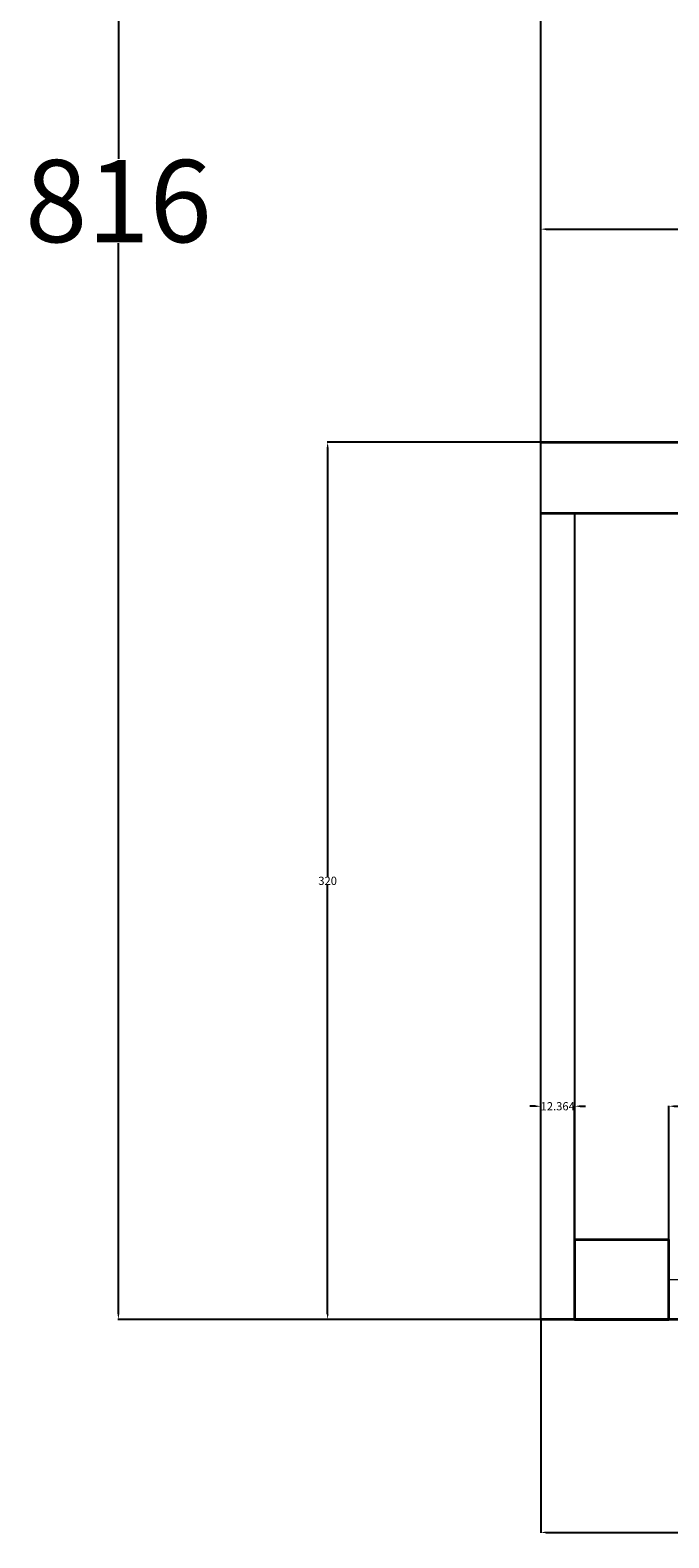
# Model space of a CAD drawing. Units: centimetres. Extents: x -121 to 3851, y -16 to 1180.
# Tile 10 of 16: x 2225 to 2458, y 16 to 566. Entities that reach past the tile are written whole.
import ezdxf

# ---------------------------------------------------------------- set-up
doc = ezdxf.new("R2010")
doc.units = ezdxf.units.CM
doc.header["$MEASUREMENT"] = 0
for name, color, linetype, lineweight in [('A-ANNO-DIMS', 2, 'Continuous', 18), ('A-COLS', 7, 'Continuous', 35), ('A-FLOR', 8, 'Continuous', 25), ('A-FLOR-HRAL', 4, 'Continuous', 18), ('A-WALL', 7, 'Continuous', 35)]:
    doc.layers.add(name, color=color, linetype=linetype, lineweight=lineweight)
doc.styles.get("Standard").update_dxf_attribs({"font": 'arial.ttf'})
doc.dimstyles.get("Standard").update_dxf_attribs({"dimtxt": 3, "dimasz": 2, "dimexe": 0.18, "dimexo": 0.0625, "dimgap": 0.09, "dimtad": 0, "dimtih": 1, "dimtoh": 1, "dimdec": 0, "dimzin": 0, "dimdsep": 46, "dimtxsty": 'Standard', "dimcen": 0.09, "dimadec": 0, "dimazin": 0, "dimtfac": 1, "dimtdec": 0, "dimtofl": 0, "dimtmove": 0, "dimatfit": 3, "dimfxl": 1, "dimtolj": 1, "dimtzin": 0, "dimarcsym": 0})

# ---------------------------------------------------------------- blocks, each defined once
blk = doc.blocks.new('*D13')
at = {"layer": 'A-ANNO-DIMS', "color": 0, "lineweight": -2, "transparency": 16777216}
for p, q in [((2411.2, 911.72), (2257.01, 911.72)), ((2257.19, 909.72), (2257.19, 519.13)), ((2257.19, 97.72), (2257.19, 488.32)), ((2411.2, 95.72), (2257.01, 95.72))]:
    blk.add_line(p, q, dxfattribs=at)
at = {"layer": 'A-ANNO-DIMS', "color": 0, "transparency": 16777216}
for points in [[(2256.85, 909.72), (2257.52, 909.72), (2257.19, 911.72)], [(2256.85, 97.72), (2257.52, 97.72), (2257.19, 95.72)]]:
    blk.add_solid(points, dxfattribs=at)
at = {"layer": 'Defpoints', "color": 0, "transparency": 16777216}
for p in [(2411.26, 911.72), (2257.19, 95.72), (2411.26, 95.72)]:
    blk.add_point(p, dxfattribs=at)
at = {"layer": 'A-ANNO-DIMS', "color": 0, "transparency": 16777216, "insert": (2257.19, 503.72), "char_height": 3, "attachment_point": 5}
blk.add_mtext('\\A1;{\\H10x;816}', dxfattribs=at)
blk = doc.blocks.new('POST-34X29CM')
blk.add_lwpolyline([(0, 0), (34.36, 0), (34.36, 28.96), (0, 28.96)], close=True)
blk = doc.blocks.new('*D66')
at = {"layer": 'A-ANNO-DIMS', "color": 0, "lineweight": -2, "transparency": 16777216}
for p, q in [((2411.2, 415.72), (2333.33, 415.72)), ((2333.51, 413.72), (2333.51, 257.35)), ((2333.51, 97.72), (2333.51, 254.1)), ((2411.2, 95.72), (2333.33, 95.72))]:
    blk.add_line(p, q, dxfattribs=at)
at = {"layer": 'A-ANNO-DIMS', "color": 0, "transparency": 16777216}
for points in [[(2333.18, 413.72), (2333.85, 413.72), (2333.51, 415.72)], [(2333.18, 97.72), (2333.85, 97.72), (2333.51, 95.72)]]:
    blk.add_solid(points, dxfattribs=at)
at = {"layer": 'Defpoints', "color": 0, "transparency": 16777216}
for p in [(2411.26, 415.72), (2333.51, 95.72), (2411.26, 95.72)]:
    blk.add_point(p, dxfattribs=at)
at = {"layer": 'A-ANNO-DIMS', "color": 0, "transparency": 16777216, "insert": (2333.51, 255.72), "char_height": 3, "attachment_point": 5}
blk.add_mtext('\\A1;320', dxfattribs=at)
blk = doc.blocks.new('*D67')
at = {"layer": 'A-ANNO-DIMS', "color": 0, "lineweight": -2, "transparency": 16777216}
for p, q in [((2411.26, 95.66), (2411.26, 17.79)), ((2821.26, 95.66), (2821.26, 17.79)), ((2413.26, 17.97), (2612.8, 17.97)), ((2819.26, 17.97), (2619.72, 17.97))]:
    blk.add_line(p, q, dxfattribs=at)
at = {"layer": 'A-ANNO-DIMS', "color": 0, "transparency": 16777216}
for points in [[(2413.26, 18.31), (2413.26, 17.64), (2411.26, 17.97)], [(2819.26, 18.31), (2819.26, 17.64), (2821.26, 17.97)]]:
    blk.add_solid(points, dxfattribs=at)
at = {"layer": 'Defpoints', "color": 0, "transparency": 16777216}
for p in [(2411.26, 95.72), (2821.26, 95.72), (2821.26, 17.97)]:
    blk.add_point(p, dxfattribs=at)
at = {"layer": 'A-ANNO-DIMS', "color": 0, "transparency": 16777216, "insert": (2616.26, 17.97), "char_height": 3, "attachment_point": 5}
blk.add_mtext('\\A1;410', dxfattribs=at)
blk = doc.blocks.new('*D75')
at = {"layer": 'A-ANNO-DIMS', "color": 0, "lineweight": -2, "transparency": 16777216}
for p, q in [((2409.26, 173.47), (2407.26, 173.47)), ((2411.26, 95.79), (2411.26, 173.65)), ((2423.63, 95.79), (2423.63, 173.65)), ((2425.63, 173.47), (2427.63, 173.47))]:
    blk.add_line(p, q, dxfattribs=at)
at = {"layer": 'A-ANNO-DIMS', "color": 0, "transparency": 16777216}
for points in [[(2409.26, 173.81), (2409.26, 173.14), (2411.26, 173.47)], [(2425.63, 173.81), (2425.63, 173.14), (2423.63, 173.47)]]:
    blk.add_solid(points, dxfattribs=at)
at = {"layer": 'Defpoints', "color": 0, "transparency": 16777216}
for p in [(2423.63, 173.47), (2411.26, 95.72), (2423.63, 95.72)]:
    blk.add_point(p, dxfattribs=at)
at = {"layer": 'A-ANNO-DIMS', "color": 0, "transparency": 16777216, "insert": (2417.45, 173.47), "char_height": 3, "attachment_point": 5}
blk.add_mtext('\\A1;12.364', dxfattribs=at)
blk = doc.blocks.new('*D76')
at = {"layer": 'A-ANNO-DIMS', "color": 0, "lineweight": -2, "transparency": 16777216}
for p, q in [((2457.99, 95.79), (2457.99, 173.65)), ((2459.99, 173.47), (2519.59, 173.47)), ((2591.55, 173.47), (2531.94, 173.47)), ((2593.55, 95.79), (2593.55, 173.65))]:
    blk.add_line(p, q, dxfattribs=at)
at = {"layer": 'A-ANNO-DIMS', "color": 0, "transparency": 16777216}
for points in [[(2459.99, 173.81), (2459.99, 173.14), (2457.99, 173.47)], [(2591.55, 173.81), (2591.55, 173.14), (2593.55, 173.47)]]:
    blk.add_solid(points, dxfattribs=at)
at = {"layer": 'Defpoints', "color": 0, "transparency": 16777216}
for p in [(2593.55, 173.47), (2457.99, 95.72), (2593.55, 95.72)]:
    blk.add_point(p, dxfattribs=at)
at = {"layer": 'A-ANNO-DIMS', "color": 0, "transparency": 16777216, "insert": (2525.77, 173.47), "char_height": 3, "attachment_point": 5}
blk.add_mtext('\\A1;135.56', dxfattribs=at)
blk = doc.blocks.new('*D78')
at = {"layer": 'A-ANNO-DIMS', "color": 0, "lineweight": -2, "transparency": 16777216}
for p, q in [((2411.26, 415.79), (2411.26, 493.65)), ((2413.26, 493.47), (2538, 493.47)), ((2675.4, 493.47), (2550.67, 493.47)), ((2677.4, 415.79), (2677.4, 493.65))]:
    blk.add_line(p, q, dxfattribs=at)
at = {"layer": 'A-ANNO-DIMS', "color": 0, "transparency": 16777216}
for points in [[(2413.26, 493.81), (2413.26, 493.14), (2411.26, 493.47)], [(2675.4, 493.81), (2675.4, 493.14), (2677.4, 493.47)]]:
    blk.add_solid(points, dxfattribs=at)
at = {"layer": 'Defpoints', "color": 0, "transparency": 16777216}
for p in [(2677.4, 493.47), (2411.26, 415.72), (2677.4, 415.72)]:
    blk.add_point(p, dxfattribs=at)
at = {"layer": 'A-ANNO-DIMS', "color": 0, "transparency": 16777216, "insert": (2544.33, 493.47), "char_height": 3, "attachment_point": 5}
blk.add_mtext('\\A1;266.14', dxfattribs=at)

msp = doc.modelspace()

# ---------------------------------------------------------------- linework, layer by layer
at = {"layer": 'A-FLOR'}
for p, q in [((2411.2642, 95.7228), (2411.2642, 911.7228)), ((2423.6282, 389.7228), (2423.6282, 95.7228))]:
    msp.add_line(p, q, dxfattribs=at)
at = {"layer": 'A-FLOR-HRAL'}
msp.add_line((2457.9883, 110.2005), (2593.5502, 111.1316), dxfattribs=at)
at = {"layer": 'A-WALL'}
for p, q in [((2411.2642, 415.7228), (2677.3995, 415.7228)), ((2661.5376, 389.7228), (2411.2642, 389.7228)), ((3767.2642, 95.7228), (2411.2642, 95.7228))]:
    msp.add_line(p, q, dxfattribs=at)

# ---------------------------------------------------------------- block references
at = {"layer": 'A-COLS'}
msp.add_blockref('POST-34X29CM', (2423.628, 95.7227), dxfattribs=at)

# ---------------------------------------------------------------- dimensions: what is measured, and where the dimension line sits
at = {"layer": 'A-ANNO-DIMS'}
dim = msp.add_linear_dim(base=(2257.1851, 95.7228), p1=(2411.2642, 911.7228), p2=(2411.2642, 95.7228), angle=90, text='{\\H10x;<>}', dimstyle='Standard', override={"dimclrd": 0, "dimclre": 0, "dimclrt": 0}, dxfattribs=at)
dim.commit()
dim.dimension.update_dxf_attribs({"geometry": '*D13', "text_midpoint": (2257.1851, 503.7228)})
for base, p1, p2, override, picture, middle in [((2677.3995, 493.4728), (2411.2642, 415.7228), (2677.3995, 415.7228), {"dimdec": 2, "dimlfac": 1, "dimrnd": 0, "dimzin": 0, "dimdsep": 46, "dimlunit": 2}, '*D78', (2544.3319, 493.4728)), ((2423.6282, 173.4728), (2411.2642, 95.7228), (2423.6282, 95.7228), {"dimdec": 3, "dimlfac": 1, "dimrnd": 0, "dimzin": 0, "dimdsep": 46, "dimlunit": 2}, '*D75', (2417.4462, 173.4728)), ((2593.5502, 173.4728), (2457.9883, 95.7228), (2593.5502, 95.7228), {"dimdec": 2, "dimlfac": 1, "dimrnd": 0, "dimzin": 0, "dimdsep": 46, "dimlunit": 2}, '*D76', (2525.7693, 173.4728)), ((2821.2642, 17.9728), (2411.2642, 95.7228), (2821.2642, 95.7228), {"dimdec": 0, "dimlfac": 1, "dimrnd": 0, "dimzin": 0, "dimdsep": 46, "dimlunit": 2}, '*D67', (2616.2642, 17.9728))]:
    dim = msp.add_linear_dim(base=base, p1=p1, p2=p2, dimstyle='Standard', override=override, dxfattribs=at)
    dim.commit()
    dim.dimension.update_dxf_attribs({"geometry": picture, "text_midpoint": middle})
dim = msp.add_linear_dim(base=(2333.5142, 95.7228), p1=(2411.2642, 415.7228), p2=(2411.2642, 95.7228), angle=90, dimstyle='Standard', override={"dimdec": 0, "dimlfac": 1, "dimrnd": 0, "dimzin": 0, "dimdsep": 46, "dimlunit": 2}, dxfattribs=at)
dim.commit()
dim.dimension.update_dxf_attribs({"geometry": '*D66', "text_midpoint": (2333.5142, 255.7228)})

doc.saveas('drawing.dxf')
